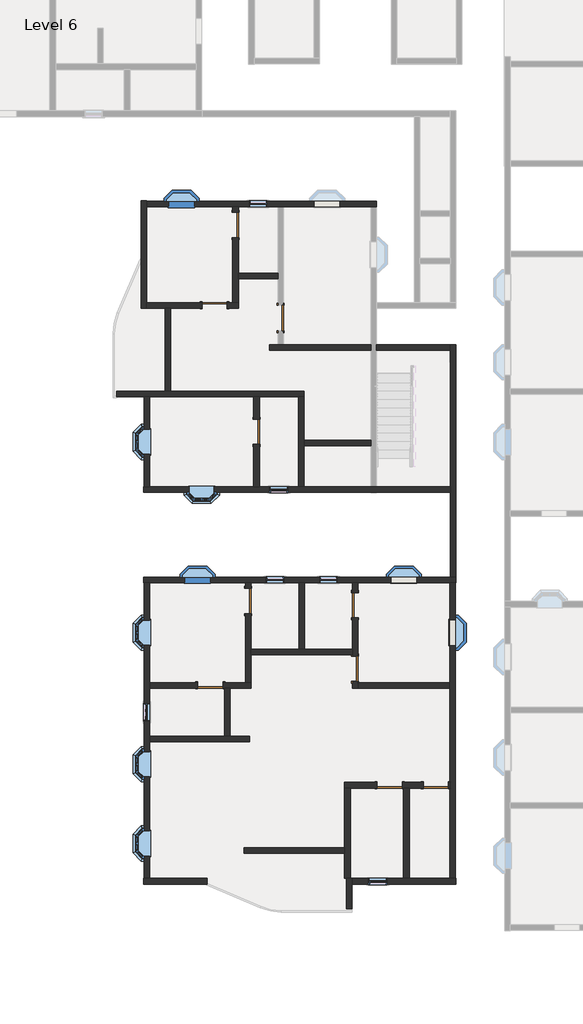
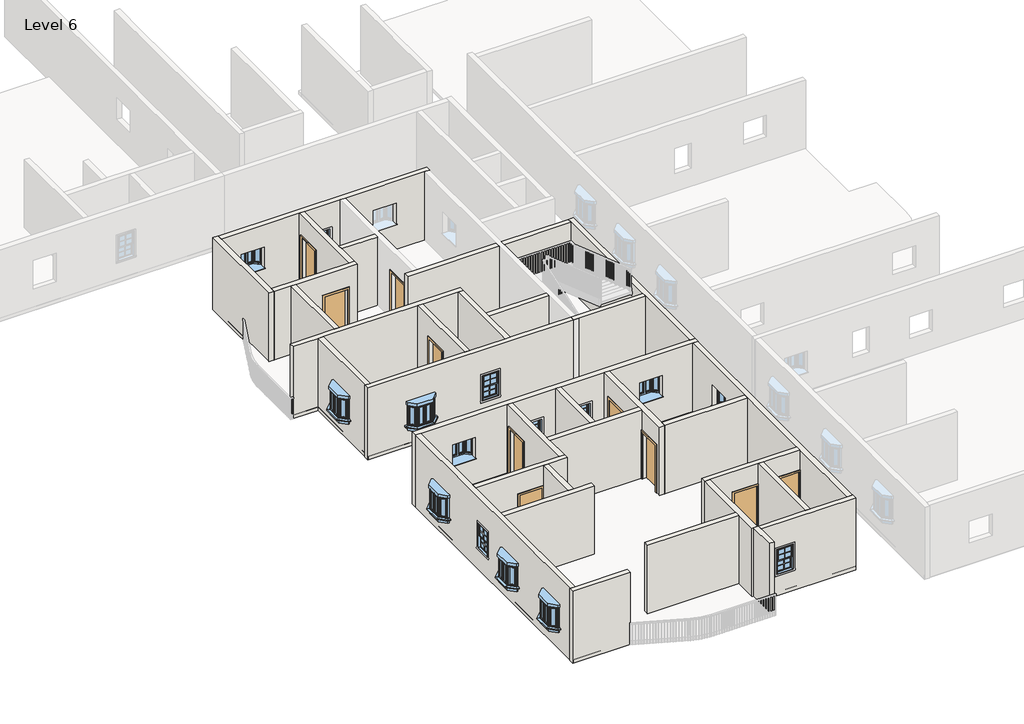
# One storey, part 1 of 14: 33 walls, 15 windows, 10 doors.
"""IFC4 building model written with IfcOpenShell, lengths in millimetres."""

from ifc_helpers import new_model, si_unit, frame, origin, place, context, project, spatial, polyline, outline, extrude, faceted_brep, transform, mapped, element, save
from components import door_54dd4da4, door_719f80de, window_910x910mm_67ef725a, window_8debb0fa

model = new_model("IFC4")

# Units and contexts
model_context = context("Model", 3, world=origin())
ifc_project = project(units=[si_unit("LENGTHUNIT", "METRE", prefix="MILLI")], contexts=[model_context])

# Site, building, storey
site = spatial("IfcSite", under=ifc_project)
building = spatial("IfcBuilding", under=site)
storey = spatial("IfcBuildingStorey", under=building, Name="Level 6", Elevation=15240.0)

# Doors
placement = place(None, origin())
door_shape = door_54dd4da4(model_context)
element("IfcDoor", 1, ObjectType="Single-Flush : 36\" x 84\"", at=placement, inside=storey, context=model_context, shape_type="MappedRepresentation", body=[
    mapped(door_shape, transform((-4626.037215, -17283.4916506, 15240.0), x_axis=(0.0, -1.0, 0.0), y_axis=(1.0, 0.0, 0.0), z_axis=(0.0, 0.0, 1.0))),
])
element("IfcDoor", 2, ObjectType="Single-Flush : 36\" x 84\"", at=placement, inside=storey, context=model_context, shape_type="MappedRepresentation", body=[
    mapped(door_shape, transform((-4626.037215, -14978.4416506, 15240.0), x_axis=(0.0, 1.0, 0.0), y_axis=(-1.0, 0.0, 0.0), z_axis=(0.0, 0.0, 1.0))),
])
element("IfcDoor", 3, ObjectType="Single-Flush : 36\" x 84\"", at=placement, inside=storey, context=model_context, shape_type="MappedRepresentation", body=[
    mapped(door_shape, transform((-9731.437215, -4100.8916506, 15240.0), x_axis=(1.0, 0.0, 0.0), y_axis=(0.0, 1.0, 0.0), z_axis=(0.0, 0.0, 1.0))),
])
element("IfcDoor", 4, ObjectType="Single-Flush : 36\" x 84\"", at=placement, inside=storey, context=model_context, shape_type="MappedRepresentation", body=[
    mapped(door_shape, transform((-7331.137215, -4558.0916506, 15240.0), x_axis=(0.0, -1.0, 0.0), y_axis=(1.0, 0.0, 0.0), z_axis=(0.0, 0.0, 1.0))),
])
door_2_shape = door_719f80de(model_context)
element("IfcDoor", 5, ObjectType="Single-Flush : 36\" x 84\"", at=placement, inside=storey, context=model_context, shape_type="MappedRepresentation", body=[
    mapped(door_2_shape, transform((-9883.837215, -17891.2072331, 15240.0), x_axis=(1.0, 0.0, 0.0), y_axis=(0.0, 1.0, 0.0), z_axis=(0.0, 0.0, 1.0))),
])
element("IfcDoor", 6, ObjectType="Single-Flush : 36\" x 84\"", at=placement, inside=storey, context=model_context, shape_type="MappedRepresentation", body=[
    mapped(door_2_shape, transform((-8512.237215, -14826.0416506, 15240.0), x_axis=(0.0, 1.0, 0.0), y_axis=(-1.0, 0.0, 0.0), z_axis=(0.0, 0.0, 1.0))),
])
element("IfcDoor", 7, ObjectType="Single-Flush : 36\" x 84\"", at=placement, inside=storey, context=model_context, shape_type="MappedRepresentation", body=[
    mapped(door_2_shape, transform((-8207.437215, -8691.9416506, 15240.0), x_axis=(0.0, 1.0, 0.0), y_axis=(-1.0, 0.0, 0.0), z_axis=(0.0, 0.0, 1.0))),
])
element("IfcDoor", 8, ObjectType="Single-Flush : 36\" x 84\"", at=placement, inside=storey, context=model_context, shape_type="MappedRepresentation", body=[
    mapped(door_2_shape, transform((-8969.437215, -1186.2416506, 15240.0), x_axis=(0.0, 1.0, 0.0), y_axis=(-1.0, 0.0, 0.0), z_axis=(0.0, 0.0, 1.0))),
])
element("IfcDoor", 9, ObjectType="Single-Flush : 36\" x 84\"", at=placement, inside=storey, context=model_context, shape_type="MappedRepresentation", body=[
    mapped(door_2_shape, transform((-3374.4891351, -21512.5916506, 15240.0), x_axis=(1.0, 0.0, 0.0), y_axis=(0.0, 1.0, 0.0), z_axis=(0.0, 0.0, 1.0))),
])
element("IfcDoor", 10, ObjectType="Single-Flush : 36\" x 84\"", at=placement, inside=storey, context=model_context, shape_type="MappedRepresentation", body=[
    mapped(door_2_shape, transform((-1698.0891351, -21512.5916506, 15240.0), x_axis=(1.0, 0.0, 0.0), y_axis=(0.0, 1.0, 0.0), z_axis=(0.0, 0.0, 1.0))),
])

# Walls
element("IfcWall", 11, ObjectType="4.5\" p", at=placement, inside=storey, context=model_context, shape_type="Brep", body=[
    faceted_brep([(-9426.637215, -17992.8072331, 17373.6), (-9426.637215, -17992.8072331, 15240.0), (-9375.837215, -17992.8072331, 15240.0), (-9172.637215, -17992.8072331, 15240.0), (-8410.637215, -17992.8072331, 15240.0), (-8410.637215, -17992.8072331, 18288.0), (-9172.637215, -17992.8072331, 18288.0), (-9375.837215, -17992.8072331, 18288.0), (-12087.287215, -17992.8072331, 18288.0), (-12087.287215, -17992.8072331, 15240.0), (-10341.037215, -17992.8072331, 15240.0), (-10341.037215, -17992.8072331, 17373.6), (-8410.637215, -17789.6072331, 15240.0), (-8613.837215, -17789.6072331, 15240.0), (-9426.637215, -17789.6072331, 15240.0), (-9426.637215, -17789.6072331, 17373.6), (-10341.037215, -17789.6072331, 17373.6), (-10341.037215, -17789.6072331, 15240.0), (-12087.287215, -17789.6072331, 15240.0), (-12087.287215, -17789.6072331, 18288.0), (-8613.837215, -17789.6072331, 18288.0), (-8410.637215, -17789.6072331, 18288.0)], [[[0, 1, 2, 3, 4, 5, 6, 7, 8, 9, 10, 11]], [[12, 13, 14, 15, 16, 17, 18, 19, 20, 21]], [[10, 9, 18, 17]], [[4, 3, 2, 1, 14, 13, 12]], [[8, 7, 6, 5, 21, 20, 19]], [[9, 8, 19, 18]], [[5, 4, 12, 21]], [[15, 14, 1, 0]], [[16, 15, 0, 11]], [[17, 16, 11, 10]]]),
])
element("IfcWall", 12, ObjectType="4.5\" p", at=placement, inside=storey, context=model_context, shape_type="Brep", body=[
    faceted_brep([(-8410.637215, -14368.8416506, 17373.6), (-8410.637215, -14368.8416506, 15240.0), (-8410.637215, -14165.6416506, 15240.0), (-8410.637215, -14165.6416506, 18288.0), (-8410.637215, -16572.2916506, 18288.0), (-8410.637215, -16775.4916506, 18288.0), (-8410.637215, -17789.6072331, 18288.0), (-8410.637215, -17789.6072331, 15240.0), (-8410.637215, -16775.4916506, 15240.0), (-8410.637215, -16572.2916506, 15240.0), (-8410.637215, -15283.2416506, 15240.0), (-8410.637215, -15283.2416506, 17373.6), (-8613.837215, -14165.6416506, 15240.0), (-8613.837215, -14368.8416506, 15240.0), (-8613.837215, -14368.8416506, 17373.6), (-8613.837215, -15283.2416506, 17373.6), (-8613.837215, -15283.2416506, 15240.0), (-8613.837215, -17789.6072331, 15240.0), (-8613.837215, -17789.6072331, 18288.0), (-8613.837215, -14165.6416506, 18288.0)], [[[0, 1, 2, 3, 4, 5, 6, 7, 8, 9, 10, 11]], [[12, 13, 14, 15, 16, 17, 18, 19]], [[2, 1, 13, 12]], [[10, 9, 8, 7, 17, 16]], [[6, 5, 4, 3, 19, 18]], [[7, 6, 18, 17]], [[3, 2, 12, 19]], [[14, 13, 1, 0]], [[15, 14, 0, 11]], [[16, 15, 11, 10]]]),
])
element("IfcWall", 13, ObjectType="4.5\" p", at=placement, inside=storey, context=model_context, shape_type="Brep", body=[
    faceted_brep([(-8410.637215, -16775.4916506, 15240.0), (-4727.637215, -16775.4916506, 15240.0), (-4727.637215, -16775.4916506, 18288.0), (-8410.637215, -16775.4916506, 18288.0), (-8410.637215, -16572.2916506, 15240.0), (-8410.637215, -16572.2916506, 18288.0), (-6670.737215, -16572.2916506, 18288.0), (-6467.537215, -16572.2916506, 18288.0), (-4727.637215, -16572.2916506, 18288.0), (-4727.637215, -16572.2916506, 15240.0), (-6467.537215, -16572.2916506, 15240.0), (-6670.737215, -16572.2916506, 15240.0)], [[[0, 1, 2, 3]], [[4, 5, 6, 7, 8, 9, 10, 11]], [[1, 0, 4, 11, 10, 9]], [[3, 2, 8, 7, 6, 5]], [[0, 3, 5, 4]], [[2, 1, 9, 8]]]),
])
element("IfcWall", 14, ObjectType="4.5\" p", at=placement, inside=storey, context=model_context, shape_type="SweptSolid", body=[
    extrude(outline(polyline([(-6670.737215, -16572.2916506), (-6670.737215, -14165.6416506), (-6467.537215, -14165.6416506), (-6467.537215, -16572.2916506), (-6670.737215, -16572.2916506)])), frame((0.0, 0.0, 15240.0), z_axis=(0.0, 0.0, 1.0), x_axis=(1.0, 0.0, 0.0)), (0.0, 0.0, 1.0), 3048.0),
])
element("IfcWall", 15, ObjectType="4.5\" p", at=placement, inside=storey, context=model_context, shape_type="Brep", body=[
    faceted_brep([(-4727.637215, -14165.6416506, 15240.0), (-4727.637215, -14521.2416506, 15240.0), (-4727.637215, -14521.2416506, 17373.6), (-4727.637215, -15435.6416506, 17373.6), (-4727.637215, -15435.6416506, 15240.0), (-4727.637215, -16572.2916506, 15240.0), (-4727.637215, -16775.4916506, 15240.0), (-4727.637215, -16826.2916506, 15240.0), (-4727.637215, -16826.2916506, 17373.6), (-4727.637215, -17740.6916506, 17373.6), (-4727.637215, -17740.6916506, 15240.0), (-4727.637215, -17994.6916506, 15240.0), (-4727.637215, -17994.6916506, 18288.0), (-4727.637215, -16775.4916506, 18288.0), (-4727.637215, -16572.2916506, 18288.0), (-4727.637215, -14165.6416506, 18288.0), (-4524.437215, -14521.2416506, 17373.6), (-4524.437215, -14521.2416506, 15240.0), (-4524.437215, -14165.6416506, 15240.0), (-4524.437215, -14165.6416506, 18288.0), (-4524.437215, -17791.4916506, 18288.0), (-4524.437215, -17994.6916506, 18288.0), (-4524.437215, -17994.6916506, 15240.0), (-4524.437215, -17791.4916506, 15240.0), (-4524.437215, -17740.6916506, 15240.0), (-4524.437215, -17740.6916506, 17373.6), (-4524.437215, -16826.2916506, 17373.6), (-4524.437215, -16826.2916506, 15240.0), (-4524.437215, -15435.6416506, 15240.0), (-4524.437215, -15435.6416506, 17373.6)], [[[0, 1, 2, 3, 4, 5, 6, 7, 8, 9, 10, 11, 12, 13, 14, 15]], [[16, 17, 18, 19, 20, 21, 22, 23, 24, 25, 26, 27, 28, 29]], [[11, 10, 24, 23, 22]], [[28, 27, 7, 6, 5, 4]], [[18, 17, 1, 0]], [[15, 14, 13, 12, 21, 20, 19]], [[0, 15, 19, 18]], [[12, 11, 22, 21]], [[25, 24, 10, 9]], [[26, 25, 9, 8]], [[27, 26, 8, 7]], [[2, 1, 17, 16]], [[3, 2, 16, 29]], [[4, 3, 29, 28]]]),
])
element("IfcWall", 16, ObjectType="4.5\" p", at=placement, inside=storey, context=model_context, shape_type="SweptSolid", body=[
    extrude(outline(polyline([(-4524.437215, -17791.4916506), (-1190.0891351, -17791.4916506), (-1190.0891351, -17994.6916506), (-4524.437215, -17994.6916506), (-4524.437215, -17791.4916506)])), frame((0.0, 0.0, 15240.0), z_axis=(0.0, 0.0, 1.0), x_axis=(1.0, 0.0, 0.0)), (0.0, 0.0, 1.0), 3048.0),
])
element("IfcWall", 17, ObjectType="4.5\" p", at=placement, inside=storey, context=model_context, shape_type="SweptSolid", body=[
    extrude(outline(polyline([(-9375.837215, -19734.5916506), (-9375.837215, -17992.8072331), (-9172.637215, -17992.8072331), (-9172.637215, -19734.5916506), (-9375.837215, -19734.5916506)])), frame((0.0, 0.0, 15240.0), z_axis=(0.0, 0.0, 1.0), x_axis=(1.0, 0.0, 0.0)), (0.0, 0.0, 1.0), 3048.0),
])
element("IfcWall", 18, ObjectType="4.5\" p", at=placement, inside=storey, context=model_context, shape_type="Brep", body=[
    faceted_brep([(-12087.287215, -19937.7916506, 15240.0), (-8455.087215, -19937.7916506, 15240.0), (-8455.087215, -19937.7916506, 18288.0), (-12087.287215, -19937.7916506, 18288.0), (-12087.287215, -19734.5916506, 15240.0), (-12087.287215, -19734.5916506, 18288.0), (-9375.837215, -19734.5916506, 18288.0), (-9172.637215, -19734.5916506, 18288.0), (-8455.087215, -19734.5916506, 18288.0), (-8455.087215, -19734.5916506, 15240.0), (-9172.637215, -19734.5916506, 15240.0), (-9375.837215, -19734.5916506, 15240.0)], [[[0, 1, 2, 3]], [[4, 5, 6, 7, 8, 9, 10, 11]], [[1, 0, 4, 11, 10, 9]], [[2, 1, 9, 8]], [[3, 2, 8, 7, 6, 5]], [[0, 3, 5, 4]]]),
])
element("IfcWall", 19, ObjectType="4.5\" p", at=placement, inside=storey, context=model_context, shape_type="Brep", body=[
    faceted_brep([(-13293.787215, -7421.9416506, 15240.0), (-12290.487215, -7421.9416506, 15240.0), (-12087.287215, -7421.9416506, 15240.0), (-8309.037215, -7421.9416506, 15240.0), (-8105.837215, -7421.9416506, 15240.0), (-6689.787215, -7421.9416506, 15240.0), (-6486.587215, -7421.9416506, 15240.0), (-6486.587215, -7421.9416506, 18288.0), (-6689.787215, -7421.9416506, 18288.0), (-8105.837215, -7421.9416506, 18288.0), (-8309.037215, -7421.9416506, 18288.0), (-12087.287215, -7421.9416506, 18288.0), (-12290.487215, -7421.9416506, 18288.0), (-13293.787215, -7421.9416506, 18288.0), (-13293.787215, -7218.7416506, 15240.0), (-13293.787215, -7218.7416506, 18288.0), (-11528.487215, -7218.7416506, 18288.0), (-11325.287215, -7218.7416506, 18288.0), (-6486.587215, -7218.7416506, 18288.0), (-6486.587215, -7218.7416506, 15240.0), (-11325.287215, -7218.7416506, 15240.0), (-11528.487215, -7218.7416506, 15240.0)], [[[0, 1, 2, 3, 4, 5, 6, 7, 8, 9, 10, 11, 12, 13]], [[14, 15, 16, 17, 18, 19, 20, 21]], [[6, 5, 4, 3, 2, 1, 0, 14, 21, 20, 19]], [[13, 12, 11, 10, 9, 8, 7, 18, 17, 16, 15]], [[0, 13, 15, 14]], [[7, 6, 19, 18]]]),
])
element("IfcWall", 20, ObjectType="4.5\" p", at=placement, inside=storey, context=model_context, shape_type="Brep", body=[
    faceted_brep([(-12201.587215, -4202.4916506, 15240.0), (-12201.587215, -3999.2916506, 15240.0), (-12201.587215, -525.8416506, 15240.0), (-12201.587215, -322.6416506, 15240.0), (-12201.587215, -309.9416506, 15240.0), (-12201.587215, -309.9416506, 18288.0), (-12201.587215, -322.6416506, 18288.0), (-12201.587215, -525.8416506, 18288.0), (-12201.587215, -3999.2916506, 18288.0), (-12201.587215, -4202.4916506, 18288.0), (-12404.787215, -4202.4916506, 15240.0), (-12404.787215, -4202.4916506, 18288.0), (-12404.787215, -309.9416506, 18288.0), (-12404.787215, -309.9416506, 15240.0)], [[[0, 1, 2, 3, 4, 5, 6, 7, 8, 9]], [[10, 11, 12, 13]], [[4, 3, 2, 1, 0, 10, 13]], [[5, 4, 13, 12]], [[9, 8, 7, 6, 5, 12, 11]], [[0, 9, 11, 10]]]),
])
element("IfcWall", 21, ObjectType="4.5\" p", at=placement, inside=storey, context=model_context, shape_type="Brep", body=[
    faceted_brep([(-9274.237215, -4202.4916506, 17373.6), (-9274.237215, -4202.4916506, 15240.0), (-8867.837215, -4202.4916506, 15240.0), (-8867.837215, -4202.4916506, 18288.0), (-11325.287215, -4202.4916506, 18288.0), (-11528.487215, -4202.4916506, 18288.0), (-12201.587215, -4202.4916506, 18288.0), (-12201.587215, -4202.4916506, 15240.0), (-11528.487215, -4202.4916506, 15240.0), (-11325.287215, -4202.4916506, 15240.0), (-10188.637215, -4202.4916506, 15240.0), (-10188.637215, -4202.4916506, 17373.6), (-8867.837215, -3999.2916506, 15240.0), (-9071.037215, -3999.2916506, 15240.0), (-9274.237215, -3999.2916506, 15240.0), (-9274.237215, -3999.2916506, 17373.6), (-10188.637215, -3999.2916506, 17373.6), (-10188.637215, -3999.2916506, 15240.0), (-12201.587215, -3999.2916506, 15240.0), (-12201.587215, -3999.2916506, 18288.0), (-9071.037215, -3999.2916506, 18288.0), (-8867.837215, -3999.2916506, 18288.0)], [[[0, 1, 2, 3, 4, 5, 6, 7, 8, 9, 10, 11]], [[12, 13, 14, 15, 16, 17, 18, 19, 20, 21]], [[2, 1, 14, 13, 12]], [[10, 9, 8, 7, 18, 17]], [[6, 5, 4, 3, 21, 20, 19]], [[7, 6, 19, 18]], [[3, 2, 12, 21]], [[15, 14, 1, 0]], [[16, 15, 0, 11]], [[17, 16, 11, 10]]]),
])
element("IfcWall", 22, ObjectType="4.5\" p", at=placement, inside=storey, context=model_context, shape_type="Brep", body=[
    faceted_brep([(-8867.837215, -729.0416506, 17373.6), (-8867.837215, -729.0416506, 15240.0), (-8867.837215, -525.8416506, 15240.0), (-8867.837215, -525.8416506, 18288.0), (-8867.837215, -2932.4916506, 18288.0), (-8867.837215, -3135.6916506, 18288.0), (-8867.837215, -3999.2916506, 18288.0), (-8867.837215, -3999.2916506, 15240.0), (-8867.837215, -3135.6916506, 15240.0), (-8867.837215, -2932.4916506, 15240.0), (-8867.837215, -1643.4416506, 15240.0), (-8867.837215, -1643.4416506, 17373.6), (-9071.037215, -525.8416506, 15240.0), (-9071.037215, -729.0416506, 15240.0), (-9071.037215, -729.0416506, 17373.6), (-9071.037215, -1643.4416506, 17373.6), (-9071.037215, -1643.4416506, 15240.0), (-9071.037215, -3999.2916506, 15240.0), (-9071.037215, -3999.2916506, 18288.0), (-9071.037215, -525.8416506, 18288.0)], [[[0, 1, 2, 3, 4, 5, 6, 7, 8, 9, 10, 11]], [[12, 13, 14, 15, 16, 17, 18, 19]], [[2, 1, 13, 12]], [[10, 9, 8, 7, 17, 16]], [[6, 5, 4, 3, 19, 18]], [[7, 6, 18, 17]], [[3, 2, 12, 19]], [[14, 13, 1, 0]], [[15, 14, 0, 11]], [[16, 15, 11, 10]]]),
])
element("IfcWall", 23, ObjectType="4.5\" p", at=placement, inside=storey, context=model_context, shape_type="SweptSolid", body=[
    extrude(outline(polyline([(-7432.737215, -3135.6916506), (-8867.837215, -3135.6916506), (-8867.837215, -2932.4916506), (-7432.737215, -2932.4916506), (-7432.737215, -3135.6916506)])), frame((0.0, 0.0, 15240.0), z_axis=(0.0, 0.0, 1.0), x_axis=(1.0, 0.0, 0.0)), (0.0, 0.0, 1.0), 3048.0),
])
element("IfcWall", 24, ObjectType="4.5\" p", at=placement, inside=storey, context=model_context, shape_type="Brep", body=[
    faceted_brep([(-7731.187215, -5726.4916506, 18288.0), (-7731.187215, -5726.4916506, 15240.0), (-4060.887215, -5726.4916506, 15240.0), (-4060.887215, -5726.4916506, 18288.0), (-7731.187215, -5523.2916506, 15240.0), (-7731.187215, -5523.2916506, 18288.0), (-7432.737215, -5523.2916506, 18288.0), (-7229.537215, -5523.2916506, 18288.0), (-4060.887215, -5523.2916506, 18288.0), (-4060.887215, -5523.2916506, 15240.0), (-7229.537215, -5523.2916506, 15240.0), (-7432.737215, -5523.2916506, 15240.0)], [[[0, 1, 2, 3]], [[4, 5, 6, 7, 8, 9, 10, 11]], [[1, 4, 11, 10, 9, 2]], [[5, 0, 3, 8, 7, 6]], [[1, 0, 5, 4]], [[3, 2, 9, 8]]]),
    faceted_brep([(-1177.3891351, -5726.4916506, 15240.0), (-1177.3891351, -5726.4916506, 18288.0), (-3857.687215, -5726.4916506, 18288.0), (-3857.687215, -5726.4916506, 15240.0), (-1177.3891351, -5523.2916506, 18288.0), (-1177.3891351, -5523.2916506, 15240.0), (-3857.687215, -5523.2916506, 15240.0), (-3857.687215, -5523.2916506, 18288.0)], [[[0, 1, 2, 3]], [[4, 5, 6, 7]], [[5, 0, 3, 6]], [[1, 4, 7, 2]], [[1, 0, 5, 4]], [[3, 2, 7, 6]]]),
])
element("IfcWall", 25, ObjectType="4.5\" p", at=placement, inside=storey, context=model_context, shape_type="SweptSolid", body=[
    extrude(outline(polyline([(-11528.487215, -7218.7416506), (-11528.487215, -4202.4916506), (-11325.287215, -4202.4916506), (-11325.287215, -7218.7416506), (-11528.487215, -7218.7416506)])), frame((0.0, 0.0, 15240.0), z_axis=(0.0, 0.0, 1.0), x_axis=(1.0, 0.0, 0.0)), (0.0, 0.0, 1.0), 3048.0),
])
element("IfcWall", 26, ObjectType="4.5\" p", at=placement, inside=storey, context=model_context, shape_type="SweptSolid", body=[
    extrude(outline(polyline([(-7421.9416506, 15240.0), (-8234.7416506, 15240.0), (-8234.7416506, 17373.6), (-9149.1416506, 17373.6), (-9149.1416506, 15240.0), (-10685.8416506, 15240.0), (-10685.8416506, 18288.0), (-7421.9416506, 18288.0), (-7421.9416506, 15240.0)])), frame((-8309.037215, 0.0, 0.0), z_axis=(1.0, 0.0, 0.0), x_axis=(0.0, 1.0, 0.0)), (0.0, 0.0, 1.0), 203.2),
])
element("IfcWall", 27, ObjectType="4.5\" p", at=placement, inside=storey, context=model_context, shape_type="Brep", body=[
    faceted_brep([(-6689.787215, -7421.9416506, 15240.0), (-6689.787215, -10685.8416506, 15240.0), (-6689.787215, -10685.8416506, 18288.0), (-6689.787215, -7421.9416506, 18288.0), (-6486.587215, -7421.9416506, 15240.0), (-6486.587215, -7421.9416506, 18288.0), (-6486.587215, -8990.3916506, 18288.0), (-6486.587215, -9193.5916506, 18288.0), (-6486.587215, -10685.8416506, 18288.0), (-6486.587215, -10685.8416506, 15240.0), (-6486.587215, -9193.5916506, 15240.0), (-6486.587215, -8990.3916506, 15240.0)], [[[0, 1, 2, 3]], [[4, 5, 6, 7, 8, 9, 10, 11]], [[1, 0, 4, 11, 10, 9]], [[3, 2, 8, 7, 6, 5]], [[0, 3, 5, 4]], [[2, 1, 9, 8]]]),
])
element("IfcWall", 28, ObjectType="4.5\" p", at=placement, inside=storey, context=model_context, shape_type="SweptSolid", body=[
    extrude(outline(polyline([(-4060.887215, -9193.5916506), (-6486.587215, -9193.5916506), (-6486.587215, -8990.3916506), (-4060.887215, -8990.3916506), (-4060.887215, -9193.5916506)])), frame((0.0, 0.0, 15240.0), z_axis=(0.0, 0.0, 1.0), x_axis=(1.0, 0.0, 0.0)), (0.0, 0.0, 1.0), 3048.0),
])
element("IfcWall", 29, ObjectType="9\"", at=placement, inside=storey, context=model_context, shape_type="SweptSolid", body=[
    extrude(outline(polyline([(-5006.4391351, -23982.7416506), (-8664.637215, -23982.7416506), (-8664.637215, -23779.5416506), (-5006.4391351, -23779.5416506), (-5006.4391351, -23982.7416506)])), frame((0.0, 0.0, 15240.0), z_axis=(0.0, 0.0, 1.0), x_axis=(1.0, 0.0, 0.0)), (0.0, 0.0, 1.0), 3048.0),
])
element("IfcWall", 30, ObjectType="9\"", at=placement, inside=storey, context=model_context, shape_type="Brep", body=[
    faceted_brep([(-1190.0891351, -21410.9916506, 15240.0), (-1240.8891351, -21410.9916506, 15240.0), (-1240.8891351, -21410.9916506, 17373.6), (-2155.2891351, -21410.9916506, 17373.6), (-2155.2891351, -21410.9916506, 15240.0), (-2917.2891351, -21410.9916506, 15240.0), (-2917.2891351, -21410.9916506, 17373.6), (-3831.6891351, -21410.9916506, 17373.6), (-3831.6891351, -21410.9916506, 15240.0), (-5006.4391351, -21410.9916506, 15240.0), (-5006.4391351, -21410.9916506, 18288.0), (-1190.0891351, -21410.9916506, 18288.0), (-1240.8891351, -21614.1916506, 17373.6), (-1240.8891351, -21614.1916506, 15240.0), (-1190.0891351, -21614.1916506, 15240.0), (-1190.0891351, -21614.1916506, 18288.0), (-2663.2891351, -21614.1916506, 18288.0), (-2866.4891351, -21614.1916506, 18288.0), (-4803.2391351, -21614.1916506, 18288.0), (-5006.4391351, -21614.1916506, 18288.0), (-5006.4391351, -21614.1916506, 15240.0), (-4803.2391351, -21614.1916506, 15240.0), (-3831.6891351, -21614.1916506, 15240.0), (-3831.6891351, -21614.1916506, 17373.6), (-2917.2891351, -21614.1916506, 17373.6), (-2917.2891351, -21614.1916506, 15240.0), (-2866.4891351, -21614.1916506, 15240.0), (-2663.2891351, -21614.1916506, 15240.0), (-2155.2891351, -21614.1916506, 15240.0), (-2155.2891351, -21614.1916506, 17373.6)], [[[0, 1, 2, 3, 4, 5, 6, 7, 8, 9, 10, 11]], [[12, 13, 14, 15, 16, 17, 18, 19, 20, 21, 22, 23, 24, 25, 26, 27, 28, 29]], [[22, 21, 20, 9, 8]], [[14, 13, 1, 0]], [[28, 27, 26, 25, 5, 4]], [[11, 10, 19, 18, 17, 16, 15]], [[0, 11, 15, 14]], [[10, 9, 20, 19]], [[6, 5, 25, 24]], [[7, 6, 24, 23]], [[8, 7, 23, 22]], [[2, 1, 13, 12]], [[3, 2, 12, 29]], [[4, 3, 29, 28]]]),
])
element("IfcWall", 31, ObjectType="9\"", at=placement, inside=storey, context=model_context, shape_type="Brep", body=[
    faceted_brep([(-5006.4391351, -21614.1916506, 15240.0), (-5006.4391351, -23779.5416506, 15240.0), (-5006.4391351, -23982.7416506, 15240.0), (-5006.4391351, -24897.1416506, 15240.0), (-5006.4391351, -24897.1416506, 18288.0), (-5006.4391351, -23982.7416506, 18288.0), (-5006.4391351, -23779.5416506, 18288.0), (-5006.4391351, -21614.1916506, 18288.0), (-4803.2391351, -21614.1916506, 15240.0), (-4803.2391351, -21614.1916506, 18288.0), (-4803.2391351, -24897.1416506, 18288.0), (-4803.2391351, -24897.1416506, 15240.0), (-4949.2891351, -24897.1416506, 15240.0), (-4949.2891351, -24897.1416506, 18288.0)], [[[0, 1, 2, 3, 4, 5, 6, 7]], [[8, 9, 10, 11]], [[3, 2, 1, 0, 8, 11, 12]], [[7, 6, 5, 4, 13, 10, 9]], [[0, 7, 9, 8]], [[4, 3, 12, 11, 10, 13]]]),
])
element("IfcWall", 32, ObjectType="9\"", at=placement, inside=storey, context=model_context, shape_type="SweptSolid", body=[
    extrude(outline(polyline([(-2866.4891351, -24897.1416506), (-2866.4891351, -21614.1916506), (-2663.2891351, -21614.1916506), (-2663.2891351, -24897.1416506), (-2866.4891351, -24897.1416506)])), frame((0.0, 0.0, 15240.0), z_axis=(0.0, 0.0, 1.0), x_axis=(1.0, 0.0, 0.0)), (0.0, 0.0, 1.0), 3048.0),
])
element("IfcWall", 33, ObjectType="9\"", at=placement, inside=storey, context=model_context, shape_type="SweptSolid", body=[
    extrude(outline(polyline([(-5006.4391351, -23982.7416506), (-8664.637215, -23982.7416506), (-8664.637215, -23779.5416506), (-5006.4391351, -23779.5416506), (-5006.4391351, -23982.7416506)])), frame((0.0, 0.0, 15240.0), z_axis=(0.0, 0.0, 1.0), x_axis=(1.0, 0.0, 0.0)), (0.0, 0.0, 1.0), 3048.0),
])
element("IfcWall", 34, ObjectType="9\" w", at=placement, inside=storey, context=model_context, shape_type="Brep", body=[
    faceted_brep([(-12303.187215, -14165.6416506, 15240.0), (-12290.487215, -14165.6416506, 15240.0), (-12087.287215, -14165.6416506, 15240.0), (-8613.837215, -14165.6416506, 15240.0), (-8410.637215, -14165.6416506, 15240.0), (-6670.737215, -14165.6416506, 15240.0), (-6467.537215, -14165.6416506, 15240.0), (-4727.637215, -14165.6416506, 15240.0), (-4524.437215, -14165.6416506, 15240.0), (-1190.0891351, -14165.6416506, 15240.0), (-986.8891351, -14165.6416506, 15240.0), (-961.4891351, -14165.6416506, 15240.0), (-961.4891351, -14165.6416506, 18288.0), (-986.8891351, -14165.6416506, 18288.0), (-1190.0891351, -14165.6416506, 18288.0), (-4524.437215, -14165.6416506, 18288.0), (-4727.637215, -14165.6416506, 18288.0), (-6467.537215, -14165.6416506, 18288.0), (-6670.737215, -14165.6416506, 18288.0), (-8410.637215, -14165.6416506, 18288.0), (-8613.837215, -14165.6416506, 18288.0), (-12087.287215, -14165.6416506, 18288.0), (-12290.487215, -14165.6416506, 18288.0), (-12303.187215, -14165.6416506, 18288.0), (-10805.562215, -14165.6416506, 17350.0), (-9895.562215, -14165.6416506, 17350.0), (-9895.562215, -14165.6416506, 16440.0), (-10805.562215, -14165.6416506, 16440.0), (-3312.2631751, -14165.6416506, 17350.0), (-2402.2631751, -14165.6416506, 17350.0), (-2402.2631751, -14165.6416506, 16440.0), (-3312.2631751, -14165.6416506, 16440.0), (-7870.887215, -14165.6416506, 17221.2), (-7210.487215, -14165.6416506, 17221.2), (-7210.487215, -14165.6416506, 16154.4), (-7870.887215, -14165.6416506, 16154.4), (-5927.787215, -14165.6416506, 17221.2), (-5267.387215, -14165.6416506, 17221.2), (-5267.387215, -14165.6416506, 16154.4), (-5927.787215, -14165.6416506, 16154.4), (-12303.187215, -13962.4416506, 15240.0), (-12303.187215, -13962.4416506, 18288.0), (-1177.3891351, -13962.4416506, 18288.0), (-974.1891351, -13962.4416506, 18288.0), (-961.4891351, -13962.4416506, 18288.0), (-961.4891351, -13962.4416506, 15240.0), (-974.1891351, -13962.4416506, 15240.0), (-1177.3891351, -13962.4416506, 15240.0), (-10805.562215, -13962.4416506, 17350.0), (-10805.562215, -13962.4416506, 16440.0), (-9895.562215, -13962.4416506, 16440.0), (-9895.562215, -13962.4416506, 17350.0), (-3312.2631751, -13962.4416506, 17350.0), (-3312.2631751, -13962.4416506, 16440.0), (-2402.2631751, -13962.4416506, 16440.0), (-2402.2631751, -13962.4416506, 17350.0), (-7870.887215, -13962.4416506, 17221.2), (-7870.887215, -13962.4416506, 16154.4), (-7210.487215, -13962.4416506, 16154.4), (-7210.487215, -13962.4416506, 17221.2), (-5927.787215, -13962.4416506, 17221.2), (-5927.787215, -13962.4416506, 16154.4), (-5267.387215, -13962.4416506, 16154.4), (-5267.387215, -13962.4416506, 17221.2)], [[[0, 1, 2, 3, 4, 5, 6, 7, 8, 9, 10, 11, 12, 13, 14, 15, 16, 17, 18, 19, 20, 21, 22, 23], [24, 25, 26, 27], [28, 29, 30, 31], [32, 33, 34, 35], [36, 37, 38, 39]], [[40, 41, 42, 43, 44, 45, 46, 47], [48, 49, 50, 51], [52, 53, 54, 55], [56, 57, 58, 59], [60, 61, 62, 63]], [[11, 10, 9, 8, 7, 6, 5, 4, 3, 2, 1, 0, 40, 47, 46, 45]], [[12, 11, 45, 44]], [[23, 22, 21, 20, 19, 18, 17, 16, 15, 14, 13, 12, 44, 43, 42, 41]], [[0, 23, 41, 40]], [[49, 48, 24, 27]], [[50, 49, 27, 26]], [[51, 50, 26, 25]], [[48, 51, 25, 24]], [[53, 52, 28, 31]], [[54, 53, 31, 30]], [[55, 54, 30, 29]], [[52, 55, 29, 28]], [[57, 56, 32, 35]], [[58, 57, 35, 34]], [[59, 58, 34, 33]], [[56, 59, 33, 32]], [[61, 60, 36, 39]], [[62, 61, 39, 38]], [[63, 62, 38, 37]], [[60, 63, 37, 36]]]),
])
element("IfcWall", 35, ObjectType="9\" w", at=placement, inside=storey, context=model_context, shape_type="Brep", body=[
    faceted_brep([(-10004.0323936, -24897.1416506, 15240.0), (-12087.287215, -24897.1416506, 15240.0), (-12290.487215, -24897.1416506, 15240.0), (-12303.187215, -24897.1416506, 15240.0), (-12303.187215, -24897.1416506, 18288.0), (-12290.487215, -24897.1416506, 18288.0), (-12087.287215, -24897.1416506, 18288.0), (-10004.0323936, -24897.1416506, 18288.0), (-10004.0323936, -25100.3416506, 15240.0), (-10004.0323936, -25100.3416506, 18288.0), (-12303.187215, -25100.3416506, 18288.0), (-12303.187215, -25100.3416506, 15240.0)], [[[0, 1, 2, 3, 4, 5, 6, 7]], [[8, 9, 10, 11]], [[3, 2, 1, 0, 8, 11]], [[4, 3, 11, 10]], [[7, 6, 5, 4, 10, 9]], [[0, 7, 9, 8]]]),
])
element("IfcWall", 36, ObjectType="9\" w", at=placement, inside=storey, context=model_context, shape_type="Brep", body=[
    faceted_brep([(-4746.0891351, -25989.3416506, 15240.0), (-4746.0891351, -25100.3416506, 15240.0), (-4746.0891351, -24897.1416506, 15240.0), (-4746.0891351, -24897.1416506, 18288.0), (-4746.0891351, -25100.3416506, 18288.0), (-4746.0891351, -25989.3416506, 18288.0), (-4949.2891351, -25989.3416506, 15240.0), (-4949.2891351, -25989.3416506, 18288.0), (-4949.2891351, -24897.1416506, 18288.0), (-4949.2891351, -24897.1416506, 15240.0), (-4803.2391351, -24897.1416506, 15240.0), (-4803.2391351, -24897.1416506, 18288.0)], [[[0, 1, 2, 3, 4, 5]], [[6, 7, 8, 9]], [[2, 1, 0, 6, 9, 10]], [[5, 4, 3, 11, 8, 7]], [[0, 5, 7, 6]], [[3, 2, 10, 9, 8, 11]]]),
])
element("IfcWall", 37, ObjectType="9\" w", at=placement, inside=storey, context=model_context, shape_type="Brep", body=[
    faceted_brep([(-4746.0891351, -25100.3416506, 15240.0), (-961.4891351, -25100.3416506, 15240.0), (-961.4891351, -25100.3416506, 18288.0), (-4746.0891351, -25100.3416506, 18288.0), (-3476.0891351, -25100.3416506, 17221.2), (-3476.0891351, -25100.3416506, 16154.4), (-4136.4891351, -25100.3416506, 16154.4), (-4136.4891351, -25100.3416506, 17221.2), (-4746.0891351, -24897.1416506, 15240.0), (-4746.0891351, -24897.1416506, 18288.0), (-2866.4891351, -24897.1416506, 18288.0), (-2663.2891351, -24897.1416506, 18288.0), (-1190.0891351, -24897.1416506, 18288.0), (-986.8891351, -24897.1416506, 18288.0), (-961.4891351, -24897.1416506, 18288.0), (-961.4891351, -24897.1416506, 15240.0), (-986.8891351, -24897.1416506, 15240.0), (-1190.0891351, -24897.1416506, 15240.0), (-2663.2891351, -24897.1416506, 15240.0), (-2866.4891351, -24897.1416506, 15240.0), (-3476.0891351, -24897.1416506, 17221.2), (-4136.4891351, -24897.1416506, 17221.2), (-4136.4891351, -24897.1416506, 16154.4), (-3476.0891351, -24897.1416506, 16154.4)], [[[0, 1, 2, 3], [4, 5, 6, 7]], [[8, 9, 10, 11, 12, 13, 14, 15, 16, 17, 18, 19], [20, 21, 22, 23]], [[1, 0, 8, 19, 18, 17, 16, 15]], [[2, 1, 15, 14]], [[3, 2, 14, 13, 12, 11, 10, 9]], [[0, 3, 9, 8]], [[5, 4, 20, 23]], [[6, 5, 23, 22]], [[7, 6, 22, 21]], [[4, 7, 21, 20]]]),
])
element("IfcWall", 38, ObjectType="9\" w", at=placement, inside=storey, context=model_context, shape_type="Brep", body=[
    faceted_brep([(-12290.487215, -14165.6416506, 15240.0), (-12290.487215, -24897.1416506, 15240.0), (-12290.487215, -24897.1416506, 18288.0), (-12290.487215, -14165.6416506, 18288.0), (-12290.487215, -16432.6244419, 17064.4), (-12290.487215, -16432.6244419, 16154.4), (-12290.487215, -15522.6244419, 16154.4), (-12290.487215, -15522.6244419, 17064.4), (-12290.487215, -21205.5916506, 17064.4), (-12290.487215, -21205.5916506, 16154.4), (-12290.487215, -20295.5916506, 16154.4), (-12290.487215, -20295.5916506, 17064.4), (-12290.487215, -24082.1416506, 17064.4), (-12290.487215, -24082.1416506, 16154.4), (-12290.487215, -23172.1416506, 16154.4), (-12290.487215, -23172.1416506, 17064.4), (-12290.487215, -19193.8994419, 17221.2), (-12290.487215, -19193.8994419, 16154.4), (-12290.487215, -18533.4994419, 16154.4), (-12290.487215, -18533.4994419, 17221.2), (-12087.287215, -14165.6416506, 15240.0), (-12087.287215, -14165.6416506, 18288.0), (-12087.287215, -17789.6072331, 18288.0), (-12087.287215, -17992.8072331, 18288.0), (-12087.287215, -19734.5916506, 18288.0), (-12087.287215, -19937.7916506, 18288.0), (-12087.287215, -24897.1416506, 18288.0), (-12087.287215, -24897.1416506, 15240.0), (-12087.287215, -19937.7916506, 15240.0), (-12087.287215, -19734.5916506, 15240.0), (-12087.287215, -17992.8072331, 15240.0), (-12087.287215, -17789.6072331, 15240.0), (-12087.287215, -16432.6244419, 17064.4), (-12087.287215, -15522.6244419, 17064.4), (-12087.287215, -15522.6244419, 16154.4), (-12087.287215, -16432.6244419, 16154.4), (-12087.287215, -21205.5916506, 17064.4), (-12087.287215, -20295.5916506, 17064.4), (-12087.287215, -20295.5916506, 16154.4), (-12087.287215, -21205.5916506, 16154.4), (-12087.287215, -24082.1416506, 17064.4), (-12087.287215, -23172.1416506, 17064.4), (-12087.287215, -23172.1416506, 16154.4), (-12087.287215, -24082.1416506, 16154.4), (-12087.287215, -19193.8994419, 17221.2), (-12087.287215, -18533.4994419, 17221.2), (-12087.287215, -18533.4994419, 16154.4), (-12087.287215, -19193.8994419, 16154.4)], [[[0, 1, 2, 3], [4, 5, 6, 7], [8, 9, 10, 11], [12, 13, 14, 15], [16, 17, 18, 19]], [[20, 21, 22, 23, 24, 25, 26, 27, 28, 29, 30, 31], [32, 33, 34, 35], [36, 37, 38, 39], [40, 41, 42, 43], [44, 45, 46, 47]], [[1, 0, 20, 31, 30, 29, 28, 27]], [[3, 2, 26, 25, 24, 23, 22, 21]], [[0, 3, 21, 20]], [[2, 1, 27, 26]], [[5, 4, 32, 35]], [[6, 5, 35, 34]], [[7, 6, 34, 33]], [[4, 7, 33, 32]], [[9, 8, 36, 39]], [[10, 9, 39, 38]], [[11, 10, 38, 37]], [[8, 11, 37, 36]], [[13, 12, 40, 43]], [[14, 13, 43, 42]], [[15, 14, 42, 41]], [[12, 15, 41, 40]], [[17, 16, 44, 47]], [[18, 17, 47, 46]], [[19, 18, 46, 45]], [[16, 19, 45, 44]]]),
])
element("IfcWall", 39, ObjectType="9\" w", at=placement, inside=storey, context=model_context, shape_type="Brep", body=[
    faceted_brep([(-1190.0891351, -14165.6416506, 15240.0), (-1190.0891351, -17791.4916506, 15240.0), (-1190.0891351, -17994.6916506, 15240.0), (-1190.0891351, -21410.9916506, 15240.0), (-1190.0891351, -21614.1916506, 15240.0), (-1190.0891351, -24897.1416506, 15240.0), (-1190.0891351, -24897.1416506, 18288.0), (-1190.0891351, -21614.1916506, 18288.0), (-1190.0891351, -21410.9916506, 18288.0), (-1190.0891351, -17994.6916506, 18288.0), (-1190.0891351, -17791.4916506, 18288.0), (-1190.0891351, -14165.6416506, 18288.0), (-1190.0891351, -15523.5666506, 17350.0), (-1190.0891351, -16433.5666506, 17350.0), (-1190.0891351, -16433.5666506, 16440.0), (-1190.0891351, -15523.5666506, 16440.0), (-986.8891351, -14165.6416506, 15240.0), (-986.8891351, -14165.6416506, 18288.0), (-986.8891351, -24897.1416506, 18288.0), (-986.8891351, -24897.1416506, 15240.0), (-986.8891351, -15523.5666506, 17350.0), (-986.8891351, -15523.5666506, 16440.0), (-986.8891351, -16433.5666506, 16440.0), (-986.8891351, -16433.5666506, 17350.0)], [[[0, 1, 2, 3, 4, 5, 6, 7, 8, 9, 10, 11], [12, 13, 14, 15]], [[16, 17, 18, 19], [20, 21, 22, 23]], [[5, 4, 3, 2, 1, 0, 16, 19]], [[11, 10, 9, 8, 7, 6, 18, 17]], [[0, 11, 17, 16]], [[6, 5, 19, 18]], [[21, 20, 12, 15]], [[22, 21, 15, 14]], [[23, 22, 14, 13]], [[20, 23, 13, 12]]]),
])
element("IfcWall", 40, ObjectType="9\" w", at=placement, inside=storey, context=model_context, shape_type="Brep", body=[
    faceted_brep([(-1177.3891351, -5523.2916506, 15240.0), (-1177.3891351, -5726.4916506, 15240.0), (-1177.3891351, -10685.8416506, 15240.0), (-1177.3891351, -10889.0416506, 15240.0), (-1177.3891351, -13962.4416506, 15240.0), (-1177.3891351, -13962.4416506, 18288.0), (-1177.3891351, -10889.0416506, 18288.0), (-1177.3891351, -10685.8416506, 18288.0), (-1177.3891351, -5726.4916506, 18288.0), (-1177.3891351, -5523.2916506, 18288.0), (-974.1891351, -5523.2916506, 15240.0), (-974.1891351, -5523.2916506, 18288.0), (-974.1891351, -13962.4416506, 18288.0), (-974.1891351, -13962.4416506, 15240.0)], [[[0, 1, 2, 3, 4, 5, 6, 7, 8, 9]], [[10, 11, 12, 13]], [[4, 3, 2, 1, 0, 10, 13]], [[9, 8, 7, 6, 5, 12, 11]], [[5, 4, 13, 12]], [[0, 9, 11, 10]]]),
])
element("IfcWall", 41, ObjectType="9\" w", at=placement, inside=storey, context=model_context, shape_type="Brep", body=[
    faceted_brep([(-1177.3891351, -10685.8416506, 15240.0), (-6486.587215, -10685.8416506, 15240.0), (-6689.787215, -10685.8416506, 15240.0), (-8105.837215, -10685.8416506, 15240.0), (-8309.037215, -10685.8416506, 15240.0), (-12087.287215, -10685.8416506, 15240.0), (-12290.487215, -10685.8416506, 15240.0), (-12303.187215, -10685.8416506, 15240.0), (-12303.187215, -10685.8416506, 18288.0), (-12290.487215, -10685.8416506, 18288.0), (-12087.287215, -10685.8416506, 18288.0), (-8309.037215, -10685.8416506, 18288.0), (-8105.837215, -10685.8416506, 18288.0), (-6689.787215, -10685.8416506, 18288.0), (-6486.587215, -10685.8416506, 18288.0), (-1177.3891351, -10685.8416506, 18288.0), (-9743.162215, -10685.8416506, 17064.4), (-10653.162215, -10685.8416506, 17064.4), (-10653.162215, -10685.8416506, 16154.4), (-9743.162215, -10685.8416506, 16154.4), (-7067.612215, -10685.8416506, 17221.2), (-7728.012215, -10685.8416506, 17221.2), (-7728.012215, -10685.8416506, 16154.4), (-7067.612215, -10685.8416506, 16154.4), (-1177.3891351, -10889.0416506, 15240.0), (-1177.3891351, -10889.0416506, 18288.0), (-12303.187215, -10889.0416506, 18288.0), (-12303.187215, -10889.0416506, 15240.0), (-9743.162215, -10889.0416506, 17064.4), (-9743.162215, -10889.0416506, 16154.4), (-10653.162215, -10889.0416506, 16154.4), (-10653.162215, -10889.0416506, 17064.4), (-7067.612215, -10889.0416506, 17221.2), (-7067.612215, -10889.0416506, 16154.4), (-7728.012215, -10889.0416506, 16154.4), (-7728.012215, -10889.0416506, 17221.2)], [[[0, 1, 2, 3, 4, 5, 6, 7, 8, 9, 10, 11, 12, 13, 14, 15], [16, 17, 18, 19], [20, 21, 22, 23]], [[24, 25, 26, 27], [28, 29, 30, 31], [32, 33, 34, 35]], [[7, 6, 5, 4, 3, 2, 1, 0, 24, 27]], [[8, 7, 27, 26]], [[15, 14, 13, 12, 11, 10, 9, 8, 26, 25]], [[0, 15, 25, 24]], [[29, 28, 16, 19]], [[30, 29, 19, 18]], [[31, 30, 18, 17]], [[28, 31, 17, 16]], [[33, 32, 20, 23]], [[34, 33, 23, 22]], [[35, 34, 22, 21]], [[32, 35, 21, 20]]]),
])
element("IfcWall", 42, ObjectType="9\" w", at=placement, inside=storey, context=model_context, shape_type="SweptSolid", body=[
    extrude(outline(polyline([(-10685.8416506, 15240.0), (-10685.8416506, 18288.0), (-7421.9416506, 18288.0), (-7421.9416506, 15240.0), (-10685.8416506, 15240.0)]), holes=[polyline([(-9508.8916506, 17064.4), (-9508.8916506, 16154.4), (-8598.8916506, 16154.4), (-8598.8916506, 17064.4), (-9508.8916506, 17064.4)])]), frame((-12290.487215, 0.0, 0.0), z_axis=(1.0, 0.0, 0.0), x_axis=(0.0, 1.0, 0.0)), (0.0, 0.0, 1.0), 203.2),
])
element("IfcWall", 43, ObjectType="9\" w", at=placement, inside=storey, context=model_context, shape_type="Brep", body=[
    faceted_brep([(-12201.587215, -525.8416506, 15240.0), (-9071.037215, -525.8416506, 15240.0), (-8867.837215, -525.8416506, 15240.0), (-7432.737215, -525.8416506, 15240.0), (-7229.537215, -525.8416506, 15240.0), (-4060.887215, -525.8416506, 15240.0), (-3857.687215, -525.8416506, 15240.0), (-3844.987215, -525.8416506, 15240.0), (-3844.987215, -525.8416506, 18288.0), (-3857.687215, -525.8416506, 18288.0), (-4060.887215, -525.8416506, 18288.0), (-7229.537215, -525.8416506, 18288.0), (-7432.737215, -525.8416506, 18288.0), (-8867.837215, -525.8416506, 18288.0), (-9071.037215, -525.8416506, 18288.0), (-12201.587215, -525.8416506, 18288.0), (-6100.212215, -525.8416506, 17350.0), (-5190.212215, -525.8416506, 17350.0), (-5190.212215, -525.8416506, 16440.0), (-6100.212215, -525.8416506, 16440.0), (-11386.587215, -525.8416506, 17350.0), (-10476.587215, -525.8416506, 17350.0), (-10476.587215, -525.8416506, 16440.0), (-11386.587215, -525.8416506, 16440.0), (-8480.487215, -525.8416506, 17221.2), (-7820.087215, -525.8416506, 17221.2), (-7820.087215, -525.8416506, 16154.4), (-8480.487215, -525.8416506, 16154.4), (-12201.587215, -322.6416506, 15240.0), (-12201.587215, -322.6416506, 18288.0), (-3844.987215, -322.6416506, 18288.0), (-3844.987215, -322.6416506, 15240.0), (-6100.212215, -322.6416506, 17350.0), (-6100.212215, -322.6416506, 16440.0), (-5190.212215, -322.6416506, 16440.0), (-5190.212215, -322.6416506, 17350.0), (-11386.587215, -322.6416506, 17350.0), (-11386.587215, -322.6416506, 16440.0), (-10476.587215, -322.6416506, 16440.0), (-10476.587215, -322.6416506, 17350.0), (-8480.487215, -322.6416506, 17221.2), (-8480.487215, -322.6416506, 16154.4), (-7820.087215, -322.6416506, 16154.4), (-7820.087215, -322.6416506, 17221.2)], [[[0, 1, 2, 3, 4, 5, 6, 7, 8, 9, 10, 11, 12, 13, 14, 15], [16, 17, 18, 19], [20, 21, 22, 23], [24, 25, 26, 27]], [[28, 29, 30, 31], [32, 33, 34, 35], [36, 37, 38, 39], [40, 41, 42, 43]], [[7, 6, 5, 4, 3, 2, 1, 0, 28, 31]], [[8, 7, 31, 30]], [[15, 14, 13, 12, 11, 10, 9, 8, 30, 29]], [[0, 15, 29, 28]], [[33, 32, 16, 19]], [[34, 33, 19, 18]], [[35, 34, 18, 17]], [[32, 35, 17, 16]], [[37, 36, 20, 23]], [[38, 37, 23, 22]], [[39, 38, 22, 21]], [[36, 39, 21, 20]], [[41, 40, 24, 27]], [[42, 41, 27, 26]], [[43, 42, 26, 25]], [[40, 43, 25, 24]]]),
])

# Windows
window_910x910mm_shape = window_910x910mm_67ef725a(model_context)
element("IfcWindow", 44, ObjectType="910x910mm", at=placement, inside=storey, context=model_context, shape_type="MappedRepresentation", body=[
    mapped(window_910x910mm_shape, transform((-10361.587215, -432.6982184, 15240.0), x_axis=(1.0, 0.0, 0.0), y_axis=(0.0, 1.0, 0.0), z_axis=(0.0, 0.0, 1.0))),
])
element("IfcWindow", 45, ObjectType="910x910mm", at=placement, inside=storey, context=model_context, shape_type="MappedRepresentation", body=[
    mapped(window_910x910mm_shape, transform((-12180.4306471, -8483.8916506, 14954.4), x_axis=(0.0, 1.0, 0.0), y_axis=(-1.0, 0.0, 0.0), z_axis=(0.0, 0.0, 1.0))),
])
element("IfcWindow", 46, ObjectType="910x910mm", at=placement, inside=storey, context=model_context, shape_type="MappedRepresentation", body=[
    mapped(window_910x910mm_shape, transform((-10768.162215, -10778.9850828, 14954.4), x_axis=(-1.0, 0.0, 0.0), y_axis=(0.0, -1.0, 0.0), z_axis=(0.0, 0.0, 1.0))),
])
element("IfcWindow", 47, ObjectType="910x910mm", at=placement, inside=storey, context=model_context, shape_type="MappedRepresentation", body=[
    mapped(window_910x910mm_shape, transform((-12180.4306471, -15407.6244419, 14954.4), x_axis=(0.0, 1.0, 0.0), y_axis=(-1.0, 0.0, 0.0), z_axis=(0.0, 0.0, 1.0))),
])
element("IfcWindow", 48, ObjectType="910x910mm", at=placement, inside=storey, context=model_context, shape_type="MappedRepresentation", body=[
    mapped(window_910x910mm_shape, transform((-9780.562215, -14072.4982184, 15240.0), x_axis=(1.0, 0.0, 0.0), y_axis=(0.0, 1.0, 0.0), z_axis=(0.0, 0.0, 1.0))),
])
element("IfcWindow", 49, ObjectType="910x910mm", at=placement, inside=storey, context=model_context, shape_type="MappedRepresentation", body=[
    mapped(window_910x910mm_shape, transform((-2287.2631751, -14072.4982184, 15240.0), x_axis=(1.0, 0.0, 0.0), y_axis=(0.0, 1.0, 0.0), z_axis=(0.0, 0.0, 1.0))),
])
element("IfcWindow", 50, ObjectType="910x910mm", at=placement, inside=storey, context=model_context, shape_type="MappedRepresentation", body=[
    mapped(window_910x910mm_shape, transform((-1096.945703, -16548.5666506, 15240.0), x_axis=(0.0, -1.0, 0.0), y_axis=(1.0, 0.0, 0.0), z_axis=(0.0, 0.0, 1.0))),
])
element("IfcWindow", 51, ObjectType="910x910mm", at=placement, inside=storey, context=model_context, shape_type="MappedRepresentation", body=[
    mapped(window_910x910mm_shape, transform((-12180.4306471, -20180.5916506, 14954.4), x_axis=(0.0, 1.0, 0.0), y_axis=(-1.0, 0.0, 0.0), z_axis=(0.0, 0.0, 1.0))),
])
element("IfcWindow", 52, ObjectType="910x910mm", at=placement, inside=storey, context=model_context, shape_type="MappedRepresentation", body=[
    mapped(window_910x910mm_shape, transform((-12180.4306471, -23057.1416506, 14954.4), x_axis=(0.0, 1.0, 0.0), y_axis=(-1.0, 0.0, 0.0), z_axis=(0.0, 0.0, 1.0))),
])
window_shape = window_8debb0fa(model_context)
element("IfcWindow", 53, ObjectType="Window-Double-Hung : 26\" x 42\"", at=placement, inside=storey, context=model_context, shape_type="MappedRepresentation", body=[
    mapped(window_shape, transform((-8150.287215, -424.2416506, 15240.0), x_axis=(1.0, 0.0, 0.0), y_axis=(0.0, 1.0, 0.0), z_axis=(0.0, 0.0, 1.0))),
])
element("IfcWindow", 54, ObjectType="Window-Double-Hung : 26\" x 42\"", at=placement, inside=storey, context=model_context, shape_type="MappedRepresentation", body=[
    mapped(window_shape, transform((-7397.812215, -10787.4416506, 15240.0), x_axis=(-1.0, 0.0, 0.0), y_axis=(0.0, -1.0, 0.0), z_axis=(0.0, 0.0, 1.0))),
])
element("IfcWindow", 55, ObjectType="Window-Double-Hung : 26\" x 42\"", at=placement, inside=storey, context=model_context, shape_type="MappedRepresentation", body=[
    mapped(window_shape, transform((-7540.687215, -14064.0416506, 15240.0), x_axis=(1.0, 0.0, 0.0), y_axis=(0.0, 1.0, 0.0), z_axis=(0.0, 0.0, 1.0))),
])
element("IfcWindow", 56, ObjectType="Window-Double-Hung : 26\" x 42\"", at=placement, inside=storey, context=model_context, shape_type="MappedRepresentation", body=[
    mapped(window_shape, transform((-5597.587215, -14064.0416506, 15240.0), x_axis=(1.0, 0.0, 0.0), y_axis=(0.0, 1.0, 0.0), z_axis=(0.0, 0.0, 1.0))),
])
element("IfcWindow", 57, ObjectType="Window-Double-Hung : 26\" x 42\"", at=placement, inside=storey, context=model_context, shape_type="MappedRepresentation", body=[
    mapped(window_shape, transform((-12188.887215, -18863.6994419, 15240.0), x_axis=(0.0, 1.0, 0.0), y_axis=(-1.0, 0.0, 0.0), z_axis=(0.0, 0.0, 1.0))),
])
element("IfcWindow", 58, ObjectType="Window-Double-Hung : 26\" x 42\"", at=placement, inside=storey, context=model_context, shape_type="MappedRepresentation", body=[
    mapped(window_shape, transform((-3806.2891351, -24998.7416506, 15240.0), x_axis=(-1.0, 0.0, 0.0), y_axis=(0.0, -1.0, 0.0), z_axis=(0.0, 0.0, 1.0))),
])

save(model, "model.ifc")

# Revit data of these elements
# Type "Single-Flush : 36\" x 84\""
#   Type Mark = "1"
#   Construction Type Id = "MDOOR"
#   Assembly Code = "C1020"
#   Analytic Construction = "Metal"
#   Thickness = 0' - 2"
#   Heat Transfer Coefficient (U) = 0.651978 BTU/(h·ft²·°F)
#   Height = 7' - 0"
#   Trim Projection Ext = 0' - 1"
#   Trim Projection Int = 0' - 1"
#   Trim Width = 0' - 3"
#   Width = 3' - 0"
#   Define Thermal Properties by = 1
#   Define Thermal Properties by = 1
#   Door Material = Door - Panel
#   Frame Material = Door - Frame
#   Visual Light Transmittance = 0
#   Solar Heat Gain Coefficient = 0
#   Function = (empty or 0)
#   Wall Closure = (empty or 0)
# Type "4.5\" p"
#   Assembly Code = "B2010"
#   Layers, outside or top first: 0' - 8" no material (function 1)
# Type "9\""
#   Assembly Code = "B2010"
#   Layers, outside or top first: 0' - 8" no material (function 1)
# Type "9\" w"
#   Assembly Code = "B2010"
#   Layers, outside or top first: 0' - 8" no material (function 1)
# Type "910x910mm"
#   Type Mark = "18"
#   Operation = "UserDefined"
#   Construction Type Id = "GSP4R"
#   Keynote = "L10"
#   Analytic Construction = "1/8 in Pilkington single glazing"
#   Wrap Layers (Ext) from Ext = 0' - 4.03543"
#   Wrap Layers (Int) from Ext = 0' - 6.98819"
#   Window Board Projection = 0' - 0.98425"
#   Window Board Extention = 0' - 0.98425"
#   Visual Light Transmittance = 0.9
#   Solar Heat Gain Coefficient = 0.78
#   Heat Transfer Coefficient (U) = 0.6496 BTU/(h·ft²·°F)
#   Glazing Thickness = 0' - 0.94488"
#   DONT CHANGE - Splay Width = 0' - 7.41997"
#   Rough Width = 2' - 11.82677"
#   Rough Height = 2' - 11.82677"
#   Roof Thickness = 0' - 4.92126"
#   Roof Overhang = 0' - 1.5748"
#   Plinth Thickness = 0' - 6.88976"
#   Height = 2' - 11.82677"
#   Width = 2' - 11.82677"
#   Frame Depth = 0' - 2.55906"
#   Default Head Height = 6' - 11.07087"
#   Cill Depth = 0' - 3.44488"
#   Cavity Closer Width = 0' - 1.9685"
#   Cavity Closer Offset from Ext = 0' - 4.03543"
#   Cavity Closer Depth = 0' - 3.34646"
#   Vis - Cavity Closers = yes
#   Define Thermal Properties by = 1
#   Material Trim = Window Frame
#   Material Glass = Glass
#   Material Frame = Window Frame
#   Manufacturer = ""
#   Wall Closure = (empty or 0)
# Type "Window-Double-Hung : 26\" x 42\""
#   Type Mark = "11"
#   Fire Rating = "0.5h"
#   Construction Type Id = "DG-DR"
#   Assembly Code = "B2020100"
#   Analytic Construction = "Double glazing - domestic"
#   Wall Thickness [instance default] = 0' - 6"
#   Window Inset [instance default] = 0' - 0"
#   Visual Light Transmittance = 0.81
#   Thermal Resistance (R) = 1.8146 (h·ft²·°F)/BTU
#   Solar Heat Gain Coefficient = 0.76
#   Muntin Width = 1' - 8"
#   Muntin Height = 1' - 5 1/8"
#   Interior Wall Closure [instance default] = 0' - 1 1/2"
#   Rough Width = 2' - 2 1/2"
#   Rough Height = 3' - 6 1/2"
#   Frame Extension [instance default] = 0' - 1 1/4"
#   Exterior Wall Closure [instance default] = 0' - 0 1/2"
#   Extension Jamb [instance default] = 0' - 1 1/2"
#   Heat Transfer Coefficient (U) = 0.5511 BTU/(h·ft²·°F)
#   Height = 3' - 6"
#   Width = 2' - 2"
#   Define Thermal Properties by = 1
#   Top Muntin Visibility = yes
#   Indicator Visibility [instance default] = yes
#   Extension Jamb Visibility [instance default] = yes
#   Interior Trim Visibility [instance default] = yes
#   Exterior Trim Visibility [instance default] = yes
#   Define Thermal Properties by = 1
#   Bottom Muntin Visibility = yes
#   Muntin Pattern = Muntin Pattern_2x2 : Muntin Pattern_2x2
#   Interior Trim Material = Wood - Stained
#   Interior Trim = Trim-Window-Interior-Flat : Picture Frame
#   Exterior Trim Material = Clad - White
#   Exterior Trim = Trim-Window-Exterior-Flat : with Sill
#   Glass Panel Material = Glass
#   Exterior Frame Material = Clad - White
#   Interior Frame Material = Wood - Stained
#   Wall Closure = (empty or 0)
# Elements 1, 2, 3, 4, 5, 6, 7, 8, 9, 10 (IfcDoor, "Single-Flush : 36\" x 84\"")
#   Phase Created = New Construction
#   Materials on its faces: "Door - Frame", "Door - Panel"
# Elements 11, 12, 13, 14, 15, 16, 17, 21, 22, 23, 24, 26, 27, 28 (IfcWall, "4.5\" p")
#   Top Offset = 0' - 0"
#   Base Offset = 0' - 0"
#   wall height = 10' - 0"
#   Phase Created = New Construction
#   Base Constraint = Level 6
#   Top Constraint = Level 7
#   Materials on its faces: "Default Wall"
# Element 18 (IfcWall, "4.5\" p")
#   Top Offset = 0' - 0"
#   Base Offset = 0' - 0"
#   wall height = 10' - 0"
#   Phase Created = New Construction
#   Base Constraint = Level 6
#   Top Constraint = Level 7
#   Materials on its faces: "Default Wall", "Door - Frame"
# Element 19 (IfcWall, "4.5\" p")
#   Top Offset = 0' - 0"
#   Base Offset = 0' - 0"
#   wall height = 10' - 0"
#   Phase Created = New Construction
#   Base Constraint = Level 6
#   Top Constraint = Level 7
#   Materials on its faces: "Default Wall", "Wood - Stained"
# Element 20 (IfcWall, "4.5\" p")
#   Top Offset = 0' - 0"
#   Base Offset = 0' - 0"
#   wall height = 10' - 0"
#   Phase Created = New Construction
#   Base Constraint = Level 6
#   Top Constraint = Level 7
#   Materials on its faces: "Default Wall", "Earth"
# Element 25 (IfcWall, "4.5\" p")
#   Top Offset = 0' - 0"
#   Base Offset = 0' - 0"
#   wall height = 10' - 0"
#   Phase Created = New Construction
#   Base Constraint = Level 6
#   Top Constraint = Level 7
#   Materials on its faces: "Default Wall", "Parking Stripe"
# Elements 29, 30, 31, 32 (IfcWall, "9\"")
#   Top Offset = 0' - 0"
#   Base Offset = 0' - 0"
#   wall height = 10' - 0"
#   Phase Created = New Construction
#   Base Constraint = Level 6
#   Top Constraint = Level 7
#   Materials on its faces: "Default Wall"
# Element 33 (IfcWall, "9\"")
#   Top Offset = 0' - 0"
#   Base Offset = 0' - 0"
#   wall height = 10' - 0"
#   Phase Created = New Construction
#   Base Constraint = Level 6
#   Top Constraint = Level 7
#   Materials on its faces: "Default Wall", "Carpet (1)"
# Elements 34, 38 (IfcWall, "9\" w")
#   Top Offset = 0' - 0"
#   Base Offset = 0' - 0"
#   wall height = 10' - 0"
#   Phase Created = New Construction
#   Base Constraint = Level 6
#   Top Constraint = Level 7
#   Materials on its faces: "Default Wall", "Parking Stripe"
# Elements 35, 37 (IfcWall, "9\" w")
#   Top Offset = 0' - 0"
#   Base Offset = 0' - 0"
#   wall height = 10' - 0"
#   Phase Created = New Construction
#   Base Constraint = Level 6
#   Top Constraint = Level 7
#   Materials on its faces: "Default Wall", "Softwood, Lumber"
# Element 36 (IfcWall, "9\" w")
#   Top Offset = 0' - 0"
#   Base Offset = 0' - 0"
#   wall height = 10' - 0"
#   Phase Created = New Construction
#   Base Constraint = Level 6
#   Top Constraint = Level 7
#   Materials on its faces: "Default Wall", "Carpet (1)"
# Elements 39, 40, 43 (IfcWall, "9\" w")
#   Top Offset = 0' - 0"
#   Base Offset = 0' - 0"
#   wall height = 10' - 0"
#   Phase Created = New Construction
#   Base Constraint = Level 6
#   Top Constraint = Level 7
#   Materials on its faces: "Default Wall"
# Elements 41, 42 (IfcWall, "9\" w")
#   Top Offset = 0' - 0"
#   Base Offset = 0' - 0"
#   wall height = 10' - 0"
#   Phase Created = New Construction
#   Base Constraint = Level 6
#   Top Constraint = Level 7
#   Materials on its faces: "Default Wall", "Wood - Stained"
# Element 44 (IfcWindow, "910x910mm")
#   Mark = "315"
#   Phase Created = New Construction
#   Materials on its faces: "Window Frame", "Glass"
# Element 45 (IfcWindow, "910x910mm")
#   Mark = "317"
#   Phase Created = New Construction
#   Materials on its faces: "Window Frame", "Glass"
# Element 46 (IfcWindow, "910x910mm")
#   Mark = "318"
#   Phase Created = New Construction
#   Materials on its faces: "Window Frame", "Glass"
# Element 47 (IfcWindow, "910x910mm")
#   Mark = "319"
#   Phase Created = New Construction
#   Materials on its faces: "Window Frame", "Glass"
# Element 48 (IfcWindow, "910x910mm")
#   Mark = "320"
#   Phase Created = New Construction
#   Materials on its faces: "Window Frame", "Glass"
# Element 49 (IfcWindow, "910x910mm")
#   Mark = "321"
#   Phase Created = New Construction
#   Materials on its faces: "Window Frame", "Glass"
# Element 50 (IfcWindow, "910x910mm")
#   Mark = "322"
#   Phase Created = New Construction
#   Materials on its faces: "Window Frame", "Glass"
# Element 51 (IfcWindow, "910x910mm")
#   Mark = "323"
#   Phase Created = New Construction
#   Materials on its faces: "Window Frame", "Glass"
# Element 52 (IfcWindow, "910x910mm")
#   Mark = "324"
#   Phase Created = New Construction
#   Materials on its faces: "Window Frame", "Glass"
# Element 53 (IfcWindow, "Window-Double-Hung : 26\" x 42\"")
#   Mark = "350"
#   Window Inset = 0' - 0"
#   Interior Wall Closure = 0' - 1 1/2"
#   Frame Extension = 0' - 1 1/4"
#   Exterior Wall Closure = 0' - 0 1/2"
#   Interior Trim Visibility = yes
#   Indicator Visibility = yes
#   Exterior Trim Visibility = yes
#   Phase Created = New Construction
#   Materials on its faces: "Wood - Stained", "Glass", "Clad - White"
# Element 54 (IfcWindow, "Window-Double-Hung : 26\" x 42\"")
#   Mark = "351"
